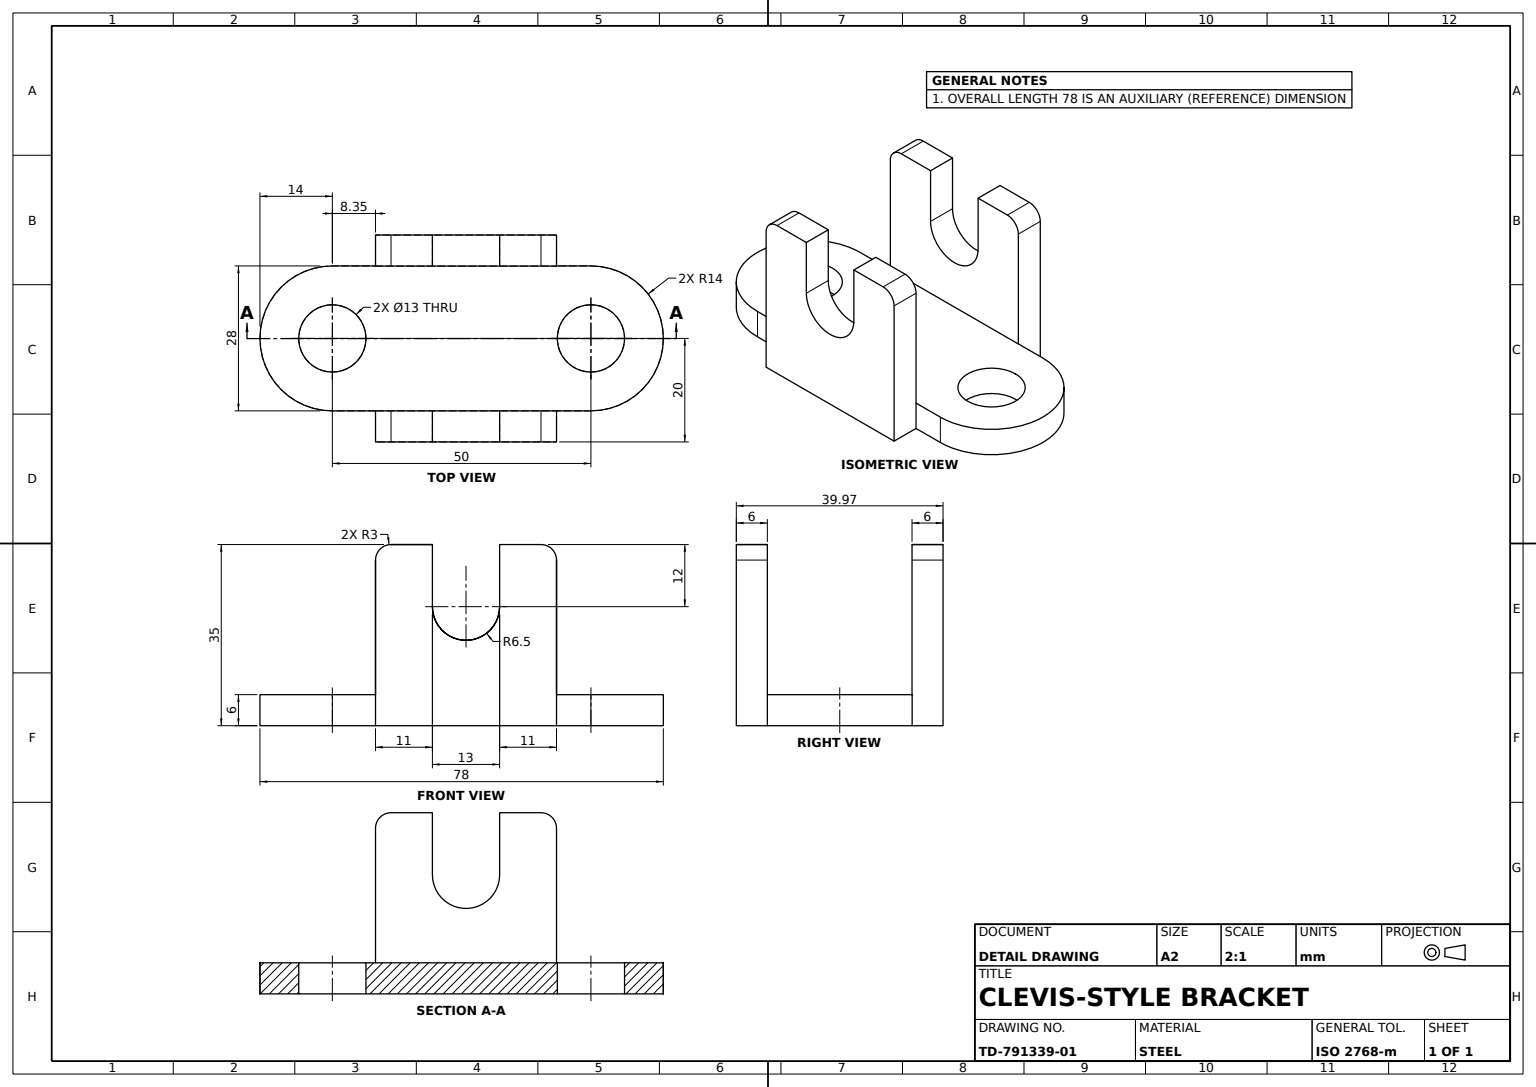
SolidWorks part; units mm, degrees
material "Plain Carbon Steel"
ref_plane "Front Plane" through (0, 0, 0) normal (0, 0, 1) x (1, 0, 0)
ref_plane "Top Plane" through (0, 0, 0) normal (0, 1, 0) x (1, 0, 0)
ref_plane "Right Plane" through (0, 0, 0) normal (1, 0, 0) x (0, 0, -1)
sketch "Clevis Ear 1 Sketch" plane through (0, 0, 0) normal (0, 0, 1) x (1, 0, 0)
  line L0 (-27.2118, 0) -> (7.7882, 0)
  line L1 (7.7882, 0) -> (7.7882, 32)
  line L2 (-27.2118, 0) -> (-27.2118, 32)
  line L3 (-24.2118, 35) -> (-16.2118, 35)
  line L5 (-3.2118, 35) -> (4.7882, 35)
  line L7 (-16.2118, 35) -> (-16.2118, 23)
  line L9 (-3.2118, 23) -> (-3.2118, 35)
  arc A0 (-16.2118, 23) -> (-3.2118, 23) centre (-9.7118, 23) ccw
  arc A1 (7.7882, 32) -> (4.7882, 35) centre (4.7882, 32) ccw
  arc A2 (-24.2118, 35) -> (-27.2118, 32) centre (-24.2118, 32) ccw
  point P14 (-27.2118, 35)
  dimension "D6" = 13
  dimension "D5" = 3
  dimension "D1" = 35
  dimension "D2" = 35
  dimension "D3" = 13
  dimension "D4" = 11
  dimension "D7" = 12
  dimension "D8" = 27.2118
extrude "Clevis Ear 1" add sketch "Clevis Ear 1 Sketch" along normal blind 6
sketch "Base Plate Sketch" plane through (0, 0, 0) normal (0, -1, 0) x (1, 0, 0)
  line L0 (-35.5584, 5.9744) -> (14.4416, 5.9744)
  line L3 (-35.5584, 33.9744) -> (14.4416, 33.9744)
  arc A0 (-35.5584, 33.9744) -> (-35.5584, 5.9744) centre (-35.5584, 19.9744) ccw
  arc A1 (14.4416, 5.9744) -> (14.4416, 33.9744) centre (14.4416, 19.9744) ccw
  dimension "D3" = 28
  dimension "D4" = 28
  dimension "D1" = 35.5584
  dimension "D2" = 19.9744
  dimension "D5" = 50
extrude "Base Plate" add sketch "Base Plate Sketch" against normal blind 6
sketch "Mounting Holes Sketch" plane through (0, 6, 0) normal (0, 1, 0) x (1, 0, 0)
  circle A0 centre (-35.5584, -19.9744) radius 6.5
  circle A1 centre (14.4416, -19.9744) radius 6.5
  dimension "D1" = 13
  dimension "D2" = 13
extrude "Mounting Holes 2xØ13" cut sketch "Mounting Holes Sketch" against normal through all
sketch "Clevis Ear 2 Sketch" plane through (0, 0, 33.9744) normal (0, 0, 1) x (1, 0, 0)
  line L0 (-27.2118, 0) -> (7.7882, 0)
  line L1 (7.7882, 0) -> (7.7882, 32)
  line L2 (4.7882, 35) -> (-3.2118, 35)
  line L4 (-16.2118, 35) -> (-24.2118, 35)
  line L5 (-27.2118, 32) -> (-27.2118, 0)
  line L6 (-16.2118, 35) -> (-16.2118, 23)
  line L8 (-3.2118, 23) -> (-3.2118, 35)
  arc A0 (-16.2118, 23) -> (-3.2118, 23) centre (-9.7118, 23) ccw
  arc A1 (7.7882, 32) -> (4.7882, 35) centre (4.7882, 32) ccw
  arc A2 (-24.2118, 35) -> (-27.2118, 32) centre (-24.2118, 32) ccw
  dimension "D1" = 3
extrude "Clevis Ear 2" add sketch "Clevis Ear 2 Sketch" along normal blind 6
